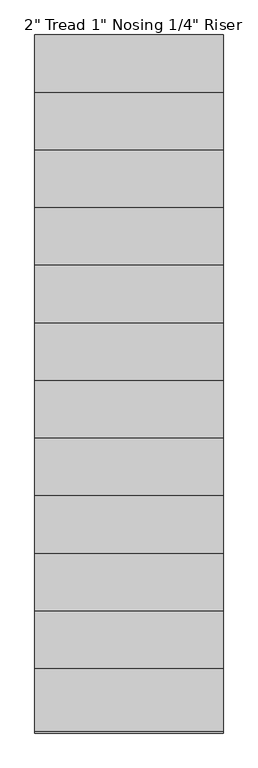
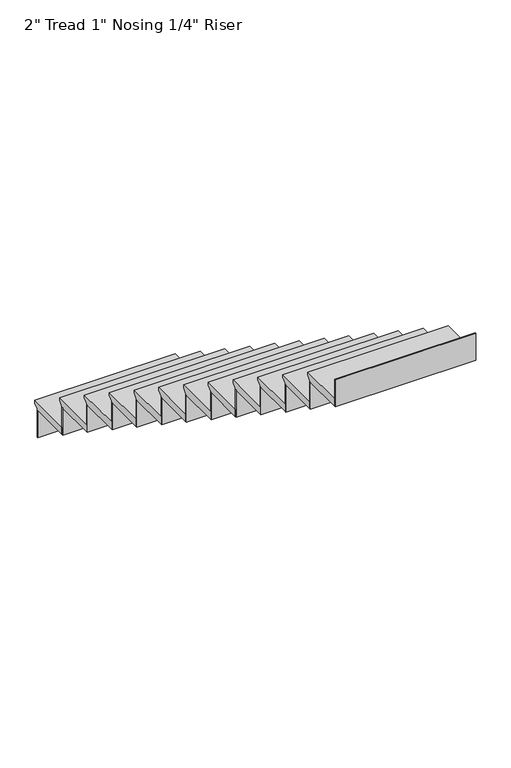
"""IFC4 building model written with IfcOpenShell, lengths in millimetres: stair flight geometry."""

from ifc_helpers import new_model, si_unit, frame, origin, place, context, project, spatial, polyline, outline, extrude, source, transform, mapped, element, save


def stair_flight_52fba82a(model_context):
    return source(origin(), model_context, "Body", "SweptSolid", [
        extrude(outline(polyline([(5429.4237487, 1870.3636364), (5734.2237487, 1870.3636364), (5734.2237487, 1851.3136364), (5708.8237487, 1825.9136364), (5708.8237487, 1819.5636364), (5429.4237487, 1819.5636364), (5429.4237487, 1870.3636364)])), frame((-6148.6994093, 0.0, 0.0), z_axis=(1.0, 0.0, 0.0), x_axis=(0.0, 1.0, 0.0)), (0.0, 0.0, 1.0), 914.4),
        extrude(outline(polyline([(-6148.6994093, 5702.4737487), (-6148.6994093, 5708.8237487), (-5234.2994093, 5708.8237487), (-5234.2994093, 5702.4737487), (-6148.6994093, 5702.4737487)])), frame((0.0, 0.0, 1632.5272727), z_axis=(0.0, 0.0, 1.0), x_axis=(1.0, 0.0, 0.0)), (0.0, 0.0, 1.0), 187.0363636),
        extrude(outline(polyline([(-6148.6994093, 5423.0737487), (-6148.6994093, 5429.4237487), (-5234.2994093, 5429.4237487), (-5234.2994093, 5423.0737487), (-6148.6994093, 5423.0737487)])), frame((0.0, 0.0, 1819.5636364), z_axis=(0.0, 0.0, 1.0), x_axis=(1.0, 0.0, 0.0)), (0.0, 0.0, 1.0), 187.0363636),
        extrude(outline(polyline([(5150.0237487, 2057.4), (5454.8237487, 2057.4), (5454.8237487, 2038.35), (5429.4237487, 2012.95), (5429.4237487, 2006.6), (5150.0237487, 2006.6), (5150.0237487, 2057.4)])), frame((-6148.6994093, 0.0, 0.0), z_axis=(1.0, 0.0, 0.0), x_axis=(0.0, 1.0, 0.0)), (0.0, 0.0, 1.0), 914.4),
        extrude(outline(polyline([(-6148.6994093, 5143.6737487), (-6148.6994093, 5150.0237487), (-5234.2994093, 5150.0237487), (-5234.2994093, 5143.6737487), (-6148.6994093, 5143.6737487)])), frame((0.0, 0.0, 2006.6), z_axis=(0.0, 0.0, 1.0), x_axis=(1.0, 0.0, 0.0)), (0.0, 0.0, 1.0), 187.0363636),
        extrude(outline(polyline([(4870.6237487, 2244.4363636), (5175.4237487, 2244.4363636), (5175.4237487, 2225.3863636), (5150.0237487, 2199.9863636), (5150.0237487, 2193.6363636), (4870.6237487, 2193.6363636), (4870.6237487, 2244.4363636)])), frame((-6148.6994093, 0.0, 0.0), z_axis=(1.0, 0.0, 0.0), x_axis=(0.0, 1.0, 0.0)), (0.0, 0.0, 1.0), 914.4),
        extrude(outline(polyline([(-6148.6994093, 4864.2737487), (-6148.6994093, 4870.6237487), (-5234.2994093, 4870.6237487), (-5234.2994093, 4864.2737487), (-6148.6994093, 4864.2737487)])), frame((0.0, 0.0, 2193.6363636), z_axis=(0.0, 0.0, 1.0), x_axis=(1.0, 0.0, 0.0)), (0.0, 0.0, 1.0), 187.0363636),
        extrude(outline(polyline([(4591.2237487, 2431.4727273), (4896.0237487, 2431.4727273), (4896.0237487, 2412.4227273), (4870.6237487, 2387.0227273), (4870.6237487, 2380.6727273), (4591.2237487, 2380.6727273), (4591.2237487, 2431.4727273)])), frame((-6148.6994093, 0.0, 0.0), z_axis=(1.0, 0.0, 0.0), x_axis=(0.0, 1.0, 0.0)), (0.0, 0.0, 1.0), 914.4),
        extrude(outline(polyline([(-6148.6994093, 4584.8737487), (-6148.6994093, 4591.2237487), (-5234.2994093, 4591.2237487), (-5234.2994093, 4584.8737487), (-6148.6994093, 4584.8737487)])), frame((0.0, 0.0, 2380.6727273), z_axis=(0.0, 0.0, 1.0), x_axis=(1.0, 0.0, 0.0)), (0.0, 0.0, 1.0), 187.0363636),
        extrude(outline(polyline([(4311.8237487, 2618.5090909), (4616.6237487, 2618.5090909), (4616.6237487, 2599.4590909), (4591.2237487, 2574.0590909), (4591.2237487, 2567.7090909), (4311.8237487, 2567.7090909), (4311.8237487, 2618.5090909)])), frame((-6148.6994093, 0.0, 0.0), z_axis=(1.0, 0.0, 0.0), x_axis=(0.0, 1.0, 0.0)), (0.0, 0.0, 1.0), 914.4),
        extrude(outline(polyline([(-6148.6994093, 4305.4737487), (-6148.6994093, 4311.8237487), (-5234.2994093, 4311.8237487), (-5234.2994093, 4305.4737487), (-6148.6994093, 4305.4737487)])), frame((0.0, 0.0, 2567.7090909), z_axis=(0.0, 0.0, 1.0), x_axis=(1.0, 0.0, 0.0)), (0.0, 0.0, 1.0), 187.0363636),
        extrude(outline(polyline([(4032.4237487, 2805.5454545), (4337.2237487, 2805.5454545), (4337.2237487, 2786.4954545), (4311.8237487, 2761.0954545), (4311.8237487, 2754.7454545), (4032.4237487, 2754.7454545), (4032.4237487, 2805.5454545)])), frame((-6148.6994093, 0.0, 0.0), z_axis=(1.0, 0.0, 0.0), x_axis=(0.0, 1.0, 0.0)), (0.0, 0.0, 1.0), 914.4),
        extrude(outline(polyline([(-6148.6994093, 4026.0737487), (-6148.6994093, 4032.4237487), (-5234.2994093, 4032.4237487), (-5234.2994093, 4026.0737487), (-6148.6994093, 4026.0737487)])), frame((0.0, 0.0, 2754.7454545), z_axis=(0.0, 0.0, 1.0), x_axis=(1.0, 0.0, 0.0)), (0.0, 0.0, 1.0), 187.0363636),
        extrude(outline(polyline([(3753.0237487, 2992.5818182), (4057.8237487, 2992.5818182), (4057.8237487, 2973.5318182), (4032.4237487, 2948.1318182), (4032.4237487, 2941.7818182), (3753.0237487, 2941.7818182), (3753.0237487, 2992.5818182)])), frame((-6148.6994093, 0.0, 0.0), z_axis=(1.0, 0.0, 0.0), x_axis=(0.0, 1.0, 0.0)), (0.0, 0.0, 1.0), 914.4),
        extrude(outline(polyline([(-6148.6994093, 3746.6737487), (-6148.6994093, 3753.0237487), (-5234.2994093, 3753.0237487), (-5234.2994093, 3746.6737487), (-6148.6994093, 3746.6737487)])), frame((0.0, 0.0, 2941.7818182), z_axis=(0.0, 0.0, 1.0), x_axis=(1.0, 0.0, 0.0)), (0.0, 0.0, 1.0), 187.0363636),
        extrude(outline(polyline([(3473.6237487, 3179.6181818), (3778.4237487, 3179.6181818), (3778.4237487, 3160.5681818), (3753.0237487, 3135.1681818), (3753.0237487, 3128.8181818), (3473.6237487, 3128.8181818), (3473.6237487, 3179.6181818)])), frame((-6148.6994093, 0.0, 0.0), z_axis=(1.0, 0.0, 0.0), x_axis=(0.0, 1.0, 0.0)), (0.0, 0.0, 1.0), 914.4),
        extrude(outline(polyline([(-6148.6994093, 3467.2737487), (-6148.6994093, 3473.6237487), (-5234.2994093, 3473.6237487), (-5234.2994093, 3467.2737487), (-6148.6994093, 3467.2737487)])), frame((0.0, 0.0, 3128.8181818), z_axis=(0.0, 0.0, 1.0), x_axis=(1.0, 0.0, 0.0)), (0.0, 0.0, 1.0), 187.0363636),
        extrude(outline(polyline([(3194.2237487, 3366.6545455), (3499.0237487, 3366.6545455), (3499.0237487, 3347.6045455), (3473.6237487, 3322.2045455), (3473.6237487, 3315.8545455), (3194.2237487, 3315.8545455), (3194.2237487, 3366.6545455)])), frame((-6148.6994093, 0.0, 0.0), z_axis=(1.0, 0.0, 0.0), x_axis=(0.0, 1.0, 0.0)), (0.0, 0.0, 1.0), 914.4),
        extrude(outline(polyline([(-6148.6994093, 3187.8737487), (-6148.6994093, 3194.2237487), (-5234.2994093, 3194.2237487), (-5234.2994093, 3187.8737487), (-6148.6994093, 3187.8737487)])), frame((0.0, 0.0, 3315.8545455), z_axis=(0.0, 0.0, 1.0), x_axis=(1.0, 0.0, 0.0)), (0.0, 0.0, 1.0), 187.0363636),
        extrude(outline(polyline([(2914.8237487, 3553.6909091), (3219.6237487, 3553.6909091), (3219.6237487, 3534.6409091), (3194.2237487, 3509.2409091), (3194.2237487, 3502.8909091), (2914.8237487, 3502.8909091), (2914.8237487, 3553.6909091)])), frame((-6148.6994093, 0.0, 0.0), z_axis=(1.0, 0.0, 0.0), x_axis=(0.0, 1.0, 0.0)), (0.0, 0.0, 1.0), 914.4),
        extrude(outline(polyline([(-6148.6994093, 2908.4737487), (-6148.6994093, 2914.8237487), (-5234.2994093, 2914.8237487), (-5234.2994093, 2908.4737487), (-6148.6994093, 2908.4737487)])), frame((0.0, 0.0, 3502.8909091), z_axis=(0.0, 0.0, 1.0), x_axis=(1.0, 0.0, 0.0)), (0.0, 0.0, 1.0), 187.0363636),
        extrude(outline(polyline([(2635.4237487, 3740.7272727), (2940.2237487, 3740.7272727), (2940.2237487, 3721.6772727), (2914.8237487, 3696.2772727), (2914.8237487, 3689.9272727), (2635.4237487, 3689.9272727), (2635.4237487, 3740.7272727)])), frame((-6148.6994093, 0.0, 0.0), z_axis=(1.0, 0.0, 0.0), x_axis=(0.0, 1.0, 0.0)), (0.0, 0.0, 1.0), 914.4),
        extrude(outline(polyline([(-6148.6994093, 2629.0737487), (-6148.6994093, 2635.4237487), (-5234.2994093, 2635.4237487), (-5234.2994093, 2629.0737487), (-6148.6994093, 2629.0737487)])), frame((0.0, 0.0, 3689.9272727), z_axis=(0.0, 0.0, 1.0), x_axis=(1.0, 0.0, 0.0)), (0.0, 0.0, 1.0), 187.0363636),
        extrude(outline(polyline([(-6148.6994093, 2349.6737487), (-6148.6994093, 2356.0237487), (-5234.2994093, 2356.0237487), (-5234.2994093, 2349.6737487), (-6148.6994093, 2349.6737487)])), frame((0.0, 0.0, 3876.9636364), z_axis=(0.0, 0.0, 1.0), x_axis=(1.0, 0.0, 0.0)), (0.0, 0.0, 1.0), 187.0363636),
        extrude(outline(polyline([(2356.0237487, 3927.7636364), (2660.8237487, 3927.7636364), (2660.8237487, 3908.7136364), (2635.4237487, 3883.3136364), (2635.4237487, 3876.9636364), (2356.0237487, 3876.9636364), (2356.0237487, 3927.7636364)])), frame((-6148.6994093, 0.0, 0.0), z_axis=(1.0, 0.0, 0.0), x_axis=(0.0, 1.0, 0.0)), (0.0, 0.0, 1.0), 914.4),
    ])


if __name__ == "__main__":
    model = new_model("IFC4")
    model_context = context("Model", 3, world=origin())
    ifc_project = project(units=[si_unit("LENGTHUNIT", "METRE", prefix="MILLI")], contexts=[model_context])
    site = spatial("IfcSite", under=ifc_project)
    building = spatial("IfcBuilding", under=site)
    placement = place(None, origin())
    stair_flight_shape = stair_flight_52fba82a(model_context)
    element("IfcStairFlight", 1, ObjectType="2\" Tread 1\" Nosing 1/4\" Riser", at=placement, inside=building, context=model_context, shape_type="MappedRepresentation", body=[
        mapped(stair_flight_shape, transform((0.0, 0.0, 0.0), x_axis=(1.0, 0.0, 0.0), y_axis=(0.0, 1.0, 0.0), z_axis=(0.0, 0.0, 1.0))),
    ])
    save(model, "model.ifc")
